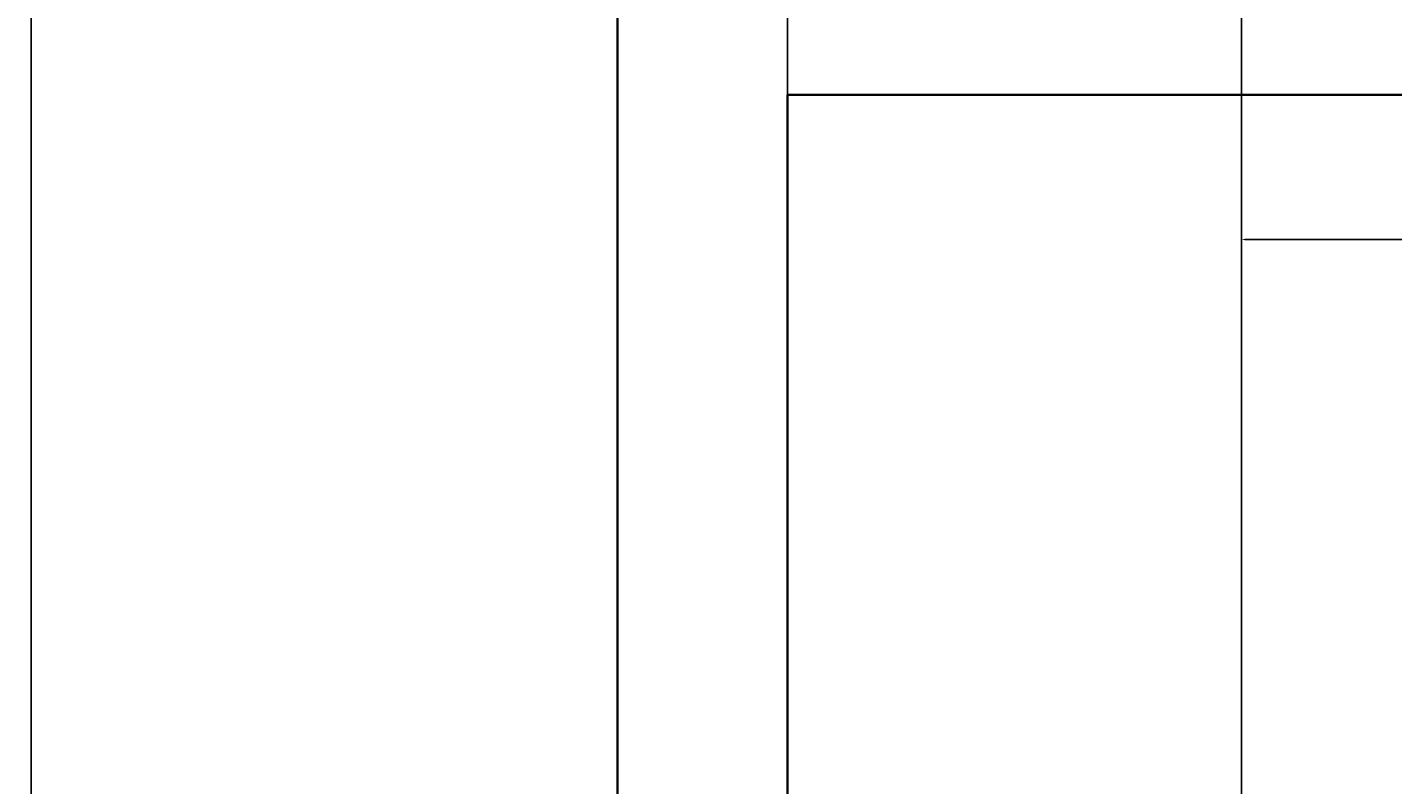
# Model space of a CAD drawing. Units: feet. Extents: x 1654 to 2985, y 1348 to 2230.
# Tile 3 of 53: x 1812 to 1884, y 1706 to 1746. Entities that reach past the tile are written whole.
import ezdxf

# ---------------------------------------------------------------- set-up
doc = ezdxf.new("R2010")
doc.units = ezdxf.units.FT
doc.layers.add('A-ANNO-DIMS', color=2, linetype='Continuous', lineweight=18)
doc.layers.add('A-WALL', color=7, linetype='Continuous', lineweight=35)
doc.styles.get("Standard").update_dxf_attribs({"font": 'arial.ttf'})
doc.dimstyles.get("Standard").update_dxf_attribs({"dimtxt": 0.18, "dimasz": 0.18, "dimexe": 0.18, "dimexo": 0.0625, "dimgap": 0.09, "dimtad": 0, "dimtih": 1, "dimtoh": 1, "dimdec": 4, "dimzin": 0, "dimdsep": 46, "dimtxsty": 'Standard', "dimcen": 0.09, "dimadec": 0, "dimazin": 0, "dimtfac": 1, "dimtdec": 4, "dimtofl": 0, "dimtmove": 0, "dimatfit": 3, "dimfxl": 1, "dimtolj": 1, "dimtzin": 0, "dimarcsym": 0})

# ---------------------------------------------------------------- blocks, each defined once
blk = doc.blocks.new('*D75')
at = {"layer": 'A-ANNO-DIMS', "color": 0, "lineweight": -2, "transparency": 16777216}
for p, q in [((1876.092, 1751.192), (1876.092, 1734.425)), ((1948.092, 1751.192), (1948.092, 1734.425)), ((1876.272, 1734.605), (1911.565, 1734.605)), ((1947.912, 1734.605), (1912.62, 1734.605))]:
    blk.add_line(p, q, dxfattribs=at)
at = {"layer": 'A-ANNO-DIMS', "color": 0, "transparency": 16777216}
for points in [[(1876.272, 1734.635), (1876.272, 1734.575), (1876.092, 1734.605)], [(1947.912, 1734.635), (1947.912, 1734.575), (1948.092, 1734.605)]]:
    blk.add_solid(points, dxfattribs=at)
at = {"layer": 'Defpoints', "color": 0, "transparency": 16777216}
for p in [(1876.092, 1751.255), (1948.092, 1751.255), (1948.092, 1734.605)]:
    blk.add_point(p, dxfattribs=at)
at = {"layer": 'A-ANNO-DIMS', "color": 0, "transparency": 16777216, "insert": (1912.092, 1734.605), "char_height": 0.18, "attachment_point": 5}
blk.add_mtext('\\A1;72 TYP.', dxfattribs=at)
blk = doc.blocks.new('*D77')
at = {"layer": 'A-ANNO-DIMS', "color": 0, "lineweight": -2, "transparency": 16777216}
for p, q in [((1843.03, 2117.255), (1811.912, 2117.255)), ((1812.092, 2117.075), (1812.092, 1841.437)), ((1812.092, 1565.435), (1812.092, 1841.073)), ((1843.03, 1565.255), (1811.912, 1565.255))]:
    blk.add_line(p, q, dxfattribs=at)
at = {"layer": 'A-ANNO-DIMS', "color": 0, "transparency": 16777216}
for points in [[(1812.062, 2117.075), (1812.122, 2117.075), (1812.092, 2117.255)], [(1812.062, 1565.435), (1812.122, 1565.435), (1812.092, 1565.255)]]:
    blk.add_solid(points, dxfattribs=at)
at = {"layer": 'Defpoints', "color": 0, "transparency": 16777216}
for p in [(1812.092, 2117.255), (1843.092, 2117.255), (1843.092, 1565.255)]:
    blk.add_point(p, dxfattribs=at)
at = {"layer": 'A-ANNO-DIMS', "color": 0, "transparency": 16777216, "insert": (1812.092, 1841.255), "char_height": 0.18, "attachment_point": 5}
blk.add_mtext('\\A1;552', dxfattribs=at)
blk = doc.blocks.new('*D100')
at = {"layer": 'A-ANNO-DIMS', "color": 0, "lineweight": -2, "transparency": 16777216}
for p, q in [((1852.092, 1751.192), (1852.092, 1534.075)), ((1876.092, 1751.192), (1876.092, 1534.075)), ((1852.272, 1534.255), (1863.872, 1534.255)), ((1875.912, 1534.255), (1864.313, 1534.255))]:
    blk.add_line(p, q, dxfattribs=at)
at = {"layer": 'A-ANNO-DIMS', "color": 0, "transparency": 16777216}
for points in [[(1852.272, 1534.285), (1852.272, 1534.225), (1852.092, 1534.255)], [(1875.912, 1534.285), (1875.912, 1534.225), (1876.092, 1534.255)]]:
    blk.add_solid(points, dxfattribs=at)
at = {"layer": 'Defpoints', "color": 0, "transparency": 16777216}
for p in [(1852.092, 1751.255), (1876.092, 1751.255), (1876.092, 1534.255)]:
    blk.add_point(p, dxfattribs=at)
at = {"layer": 'A-ANNO-DIMS', "color": 0, "transparency": 16777216, "insert": (1864.092, 1534.255), "char_height": 0.18, "attachment_point": 5}
blk.add_mtext('\\A1;24', dxfattribs=at)

msp = doc.modelspace()

# ---------------------------------------------------------------- linework, layer by layer
at = {"layer": 'A-WALL'}
for p, q in [((1843.0924, 2117.2549), (1843.0924, 1565.2549)), ((1843.0924, 1742.2549), (1843.0924, 1565.2549)), ((1852.0924, 1742.2549), (1948.0924, 1742.2549)), ((1852.0924, 1742.2549), (1852.0924, 1574.2549))]:
    msp.add_line(p, q, dxfattribs=at)

# ---------------------------------------------------------------- dimensions: what is measured, and where the dimension line sits
at = {"layer": 'A-ANNO-DIMS'}
dim = msp.add_linear_dim(base=(1812.0924, 2117.2549), p1=(1843.0924, 1565.2549), p2=(1843.0924, 2117.2549), angle=90, dimstyle='Standard', override={"dimdec": 0, "dimlfac": 1, "dimrnd": 0, "dimzin": 0, "dimdsep": 46, "dimlunit": 2}, dxfattribs=at)
dim.commit()
dim.dimension.update_dxf_attribs({"geometry": '*D77', "text_midpoint": (1812.0924, 1841.2549)})
dim = msp.add_linear_dim(base=(1876.0924, 1534.2549), p1=(1852.0924, 1751.2549), p2=(1876.0924, 1751.2549), dimstyle='Standard', override={"dimdec": 0, "dimlfac": 1, "dimrnd": 0, "dimzin": 0, "dimdsep": 46, "dimlunit": 2}, dxfattribs=at)
dim.commit()
dim.dimension.update_dxf_attribs({"geometry": '*D100', "text_midpoint": (1864.0924, 1534.2549)})
dim = msp.add_linear_dim(base=(1948.0924, 1734.6049), p1=(1876.0924, 1751.2549), p2=(1948.0924, 1751.2549), text='<> TYP.', dimstyle='Standard', override={"dimdec": 0, "dimlfac": 1, "dimrnd": 0, "dimzin": 0, "dimdsep": 46, "dimlunit": 2}, dxfattribs=at)
dim.commit()
dim.dimension.update_dxf_attribs({"geometry": '*D75', "text_midpoint": (1912.0924, 1734.6049)})

doc.saveas('drawing.dxf')
